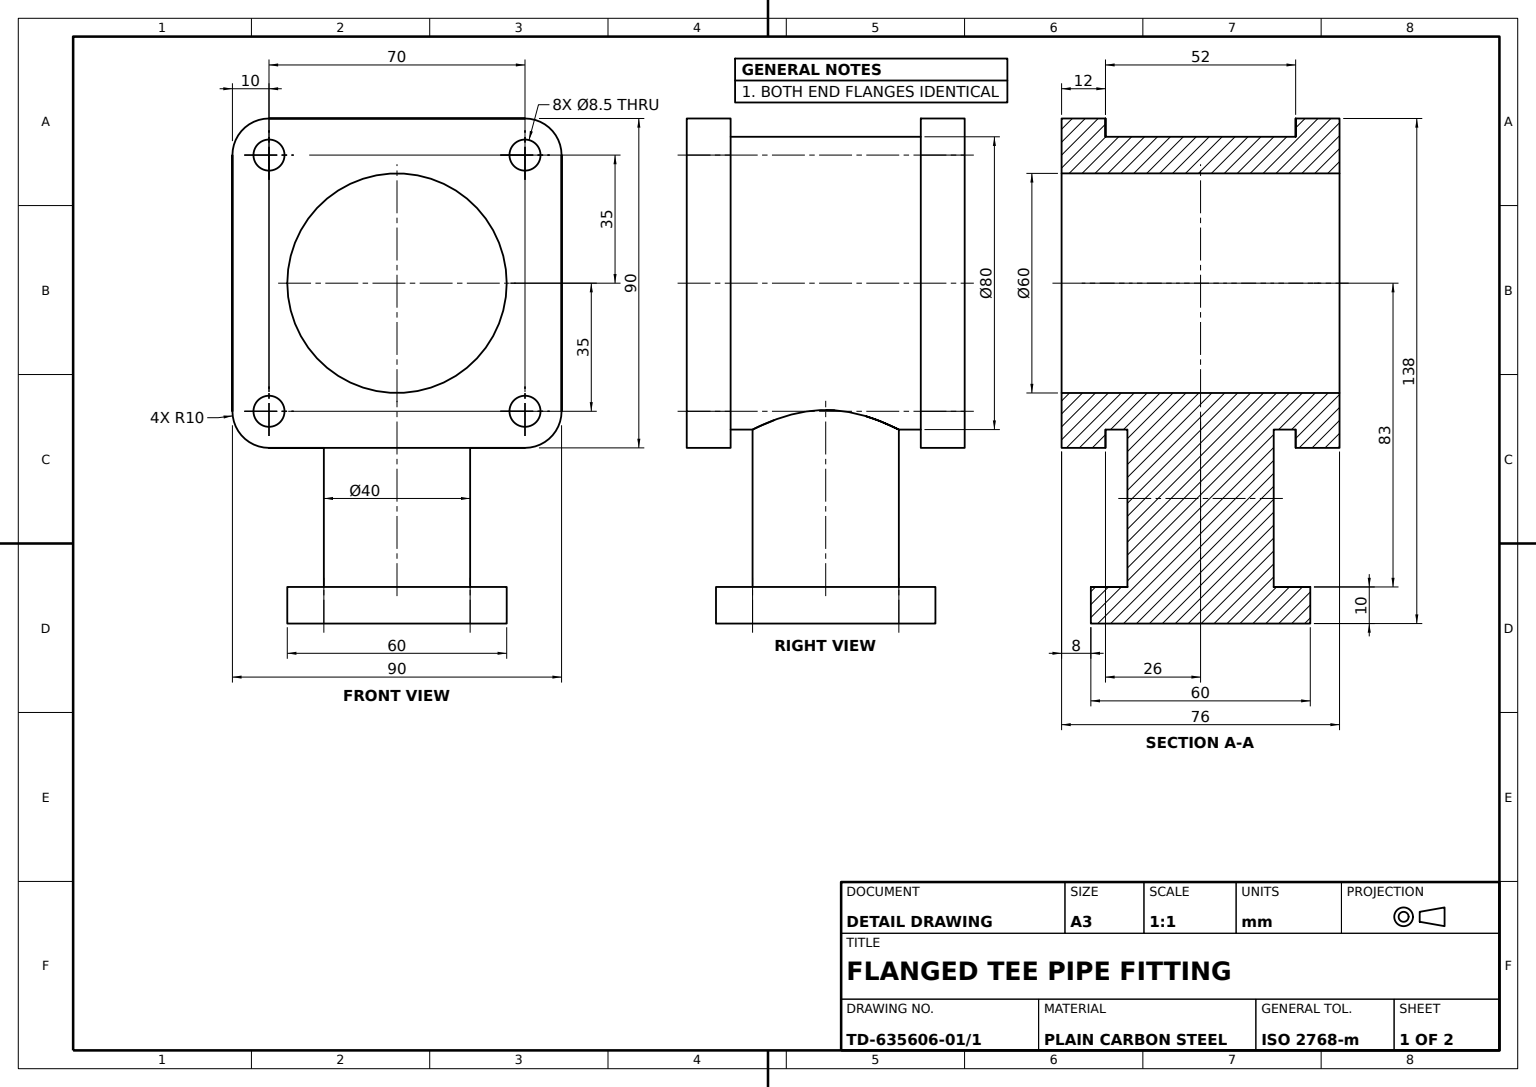
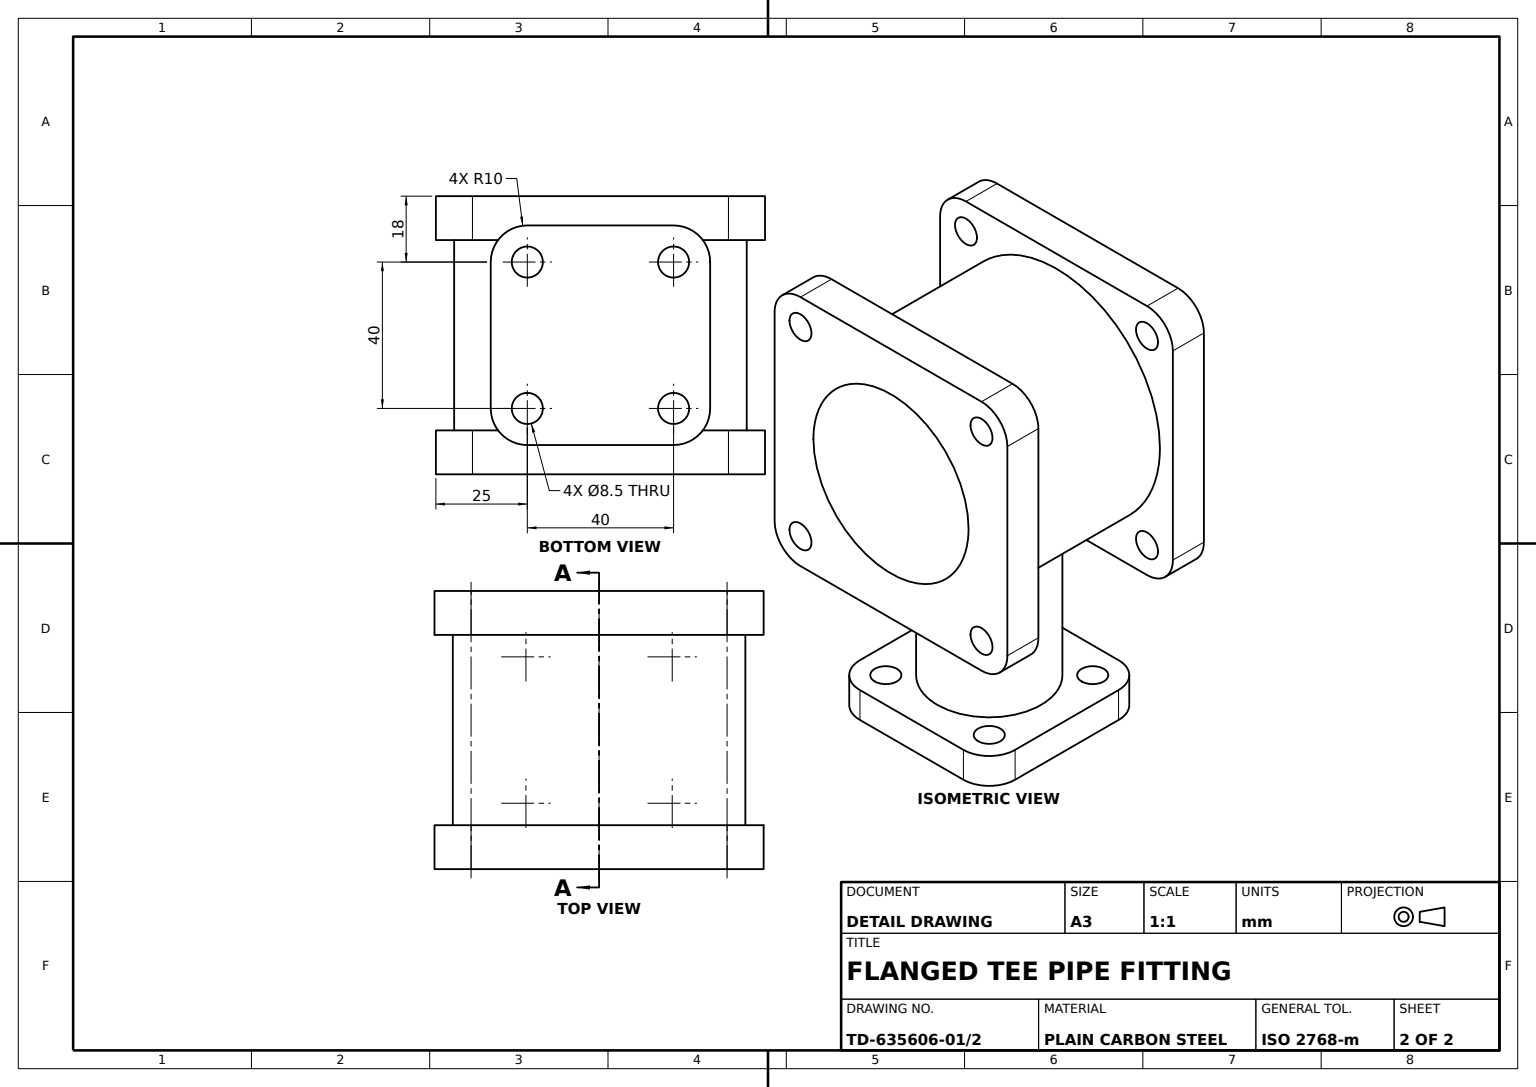
from build123d import *

# Parameters (mm, degrees)
BODY_TUBE_SKETCH_R                 = 40
BODY_TUBE_SKETCH_R_2               = 30
BODY_TUBE_80_DEPTH                 = 52
INLET_FLANGE_SKETCH_W              = 90
INLET_FLANGE_SKETCH_H              = 90
INLET_FLANGE_90X90_DEPTH           = 12
OUTLET_FLANGE_SKETCH_W             = 90
OUTLET_FLANGE_SKETCH_H             = 90
OUTLET_FLANGE_90X90_DEPTH          = 12
FLANGE_BORE_SKETCH_R               = 30
FLANGE_BORE_60_DEPTH               = 100.126182212
OUTLET_FLANGE_CORNER_FILLETS_R10_R = 10
INLET_FLANGE_CORNER_FILLETS_R10_R  = 10
INLET_FLANGE_HOLES_SKETCH_R        = 4.25
INLET_FLANGE_HOLES_4X_8_5_DEPTH    = 12
OUTLET_START                       = -12
OUTLET_FLANGE_HOLES_SKETCH_R       = 4.25
OUTLET_FLANGE_HOLES_4X_8_5_DEPTH   = 12
BRANCH_PIPE_SKETCH_R               = 20
BRANCH_PIPE_40_DEPTH               = 50
MOUNTING_FOOT_SKETCH_W             = 60
MOUNTING_FOOT_SKETCH_H             = 60
MOUNTING_FOOT_60X60_DEPTH          = 10
MOUNTING_FOOT_CORNER_FILLETS_R10_R = 10
MOUNTING_FOOT_HOLES_SKETCH_R       = 4.25
MOUNTING_FOOT_HOLES_4X_8_5_DEPTH   = 10


with BuildPart() as part:
    # Body Tube Sketch → Body Tube Ø80 (new body)
    with BuildSketch(Plane.XY):
        with Locations(Location((0, 0, 0), (0, 0, 180))):
            Circle(BODY_TUBE_SKETCH_R)
        with Locations(Location((0, 0, 0), (0, 0, 180))):
            Circle(BODY_TUBE_SKETCH_R_2, mode=Mode.SUBTRACT)
    extrude(amount=BODY_TUBE_80_DEPTH)

    # Inlet Flange Sketch → Inlet Flange 90x90 (add)
    with BuildSketch(Plane.XY):
        Rectangle(INLET_FLANGE_SKETCH_W, INLET_FLANGE_SKETCH_H)
    extrude(amount=-INLET_FLANGE_90X90_DEPTH)

    # Outlet Flange Sketch → Outlet Flange 90x90 (add)
    with BuildSketch(Plane.XY.offset(52)):
        Rectangle(OUTLET_FLANGE_SKETCH_W, OUTLET_FLANGE_SKETCH_H)
    extrude(amount=OUTLET_FLANGE_90X90_DEPTH)

    # Flange Bore Sketch → Flange Bore Ø60 (cut, through all)
    with BuildSketch(Plane.XY.offset(64)):
        with Locations(Location((0, 0, 0), (0, 0, 180))):
            Circle(FLANGE_BORE_SKETCH_R)
    extrude(amount=-FLANGE_BORE_60_DEPTH, mode=Mode.SUBTRACT)

    # Outlet Flange Corner Fillets R10
    outlet_flange_corner_fillets_r10_edges = [part.edges().sort_by_distance(p)[0] for p in [
        (45, -45, 58),
        (45, 45, 58),
        (-45, 45, 58),
        (-45, -45, 58),
    ]]
    fillet(outlet_flange_corner_fillets_r10_edges, radius=OUTLET_FLANGE_CORNER_FILLETS_R10_R)

    # Inlet Flange Corner Fillets R10
    inlet_flange_corner_fillets_r10_edges = [part.edges().sort_by_distance(p)[0] for p in [
        (-45, -45, -6),
        (-45, 45, -6),
        (45, 45, -6),
        (45, -45, -6),
    ]]
    fillet(inlet_flange_corner_fillets_r10_edges, radius=INLET_FLANGE_CORNER_FILLETS_R10_R)

    # Inlet Flange Holes Sketch → Inlet Flange Holes 4xØ8.5 (cut)
    with BuildSketch(Plane(origin=(0, 0, -12), x_dir=(-1, 0, 0), z_dir=(0, 0, -1))):
        with Locations((-35, 35)):
            Circle(INLET_FLANGE_HOLES_SKETCH_R)
        with Locations((35, 35)):
            Circle(INLET_FLANGE_HOLES_SKETCH_R)
        with Locations((35, -35)):
            Circle(INLET_FLANGE_HOLES_SKETCH_R)
        with Locations((-35, -35)):
            Circle(INLET_FLANGE_HOLES_SKETCH_R)
    extrude(amount=-INLET_FLANGE_HOLES_4X_8_5_DEPTH, mode=Mode.SUBTRACT)

    # Outlet Flange Holes Sketch → Outlet Flange Holes 4xØ8.5 (cut)
    with BuildSketch(Plane.XY.offset(64).offset(OUTLET_START)):
        with Locations(Location((-35, 35, 0), (0, 0, 180))):
            Circle(OUTLET_FLANGE_HOLES_SKETCH_R)
        with Locations(Location((35, 35, 0), (0, 0, 180))):
            Circle(OUTLET_FLANGE_HOLES_SKETCH_R)
        with Locations(Location((35, -35, 0), (0, 0, 180))):
            Circle(OUTLET_FLANGE_HOLES_SKETCH_R)
        with Locations(Location((-35, -35, 0), (0, 0, 180))):
            Circle(OUTLET_FLANGE_HOLES_SKETCH_R)
    extrude(amount=OUTLET_FLANGE_HOLES_4X_8_5_DEPTH, mode=Mode.SUBTRACT)

    # Branch Pipe Sketch → Branch Pipe Ø40 (add)
    with BuildSketch(Plane(origin=(0, -83, 0), x_dir=(1, 0, 0), z_dir=(0, 1, 0))):
        with Locations(Location((0, -26, 0), (0, 0, 90))):
            Circle(BRANCH_PIPE_SKETCH_R)
    extrude(amount=BRANCH_PIPE_40_DEPTH)

    # Mounting Foot Sketch → Mounting Foot 60x60 (add)
    with BuildSketch(Plane(origin=(0, -83, 0), x_dir=(1, 0, 0), z_dir=(0, 1, 0))):
        with Locations((0, -26)):
            Rectangle(MOUNTING_FOOT_SKETCH_W, MOUNTING_FOOT_SKETCH_H)
    extrude(amount=-MOUNTING_FOOT_60X60_DEPTH)

    # Mounting Foot Corner Fillets R10
    mounting_foot_corner_fillets_r10_edges = [part.edges().sort_by_distance(p)[0] for p in [
        (30, -88, -4),
        (30, -88, 56),
        (-30, -88, 56),
        (-30, -88, -4),
    ]]
    fillet(mounting_foot_corner_fillets_r10_edges, radius=MOUNTING_FOOT_CORNER_FILLETS_R10_R)

    # Mounting Foot Holes Sketch → Mounting Foot Holes 4xØ8.5 (cut)
    with BuildSketch(Plane.XZ.offset(93)):
        with Locations(Location((-20, 46, 0), (0, 0, 270))):
            Circle(MOUNTING_FOOT_HOLES_SKETCH_R)
        with Locations(Location((20, 46, 0), (0, 0, 270))):
            Circle(MOUNTING_FOOT_HOLES_SKETCH_R)
        with Locations(Location((20, 6, 0), (0, 0, 270))):
            Circle(MOUNTING_FOOT_HOLES_SKETCH_R)
        with Locations(Location((-20, 6, 0), (0, 0, 270))):
            Circle(MOUNTING_FOOT_HOLES_SKETCH_R)
    extrude(amount=-MOUNTING_FOOT_HOLES_4X_8_5_DEPTH, mode=Mode.SUBTRACT)


solid = part.part
